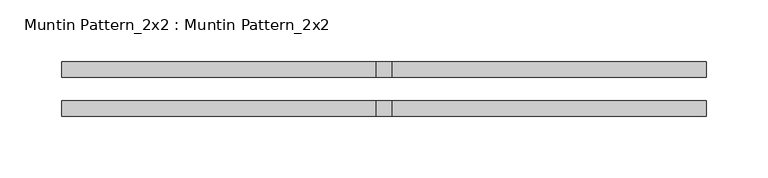
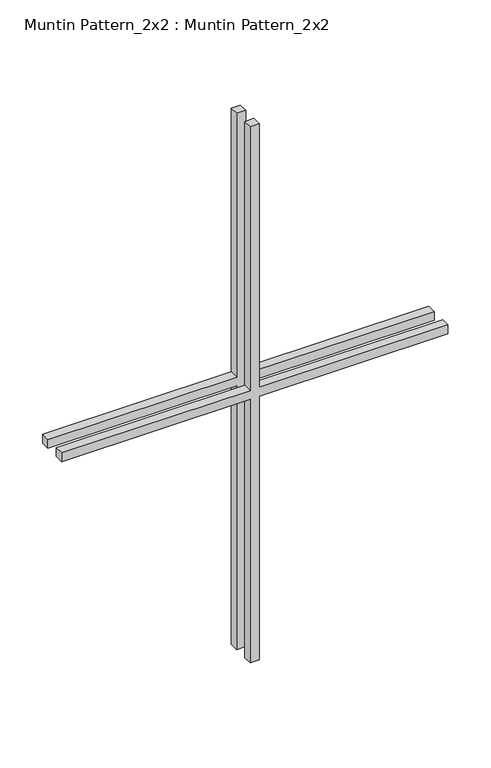
"""IFC4 building model written with IfcOpenShell, lengths in millimetres: proxy geometry, Muntin Pattern_2x2 : Muntin Pattern_2x2."""

from ifc_helpers import new_model, si_unit, frame, origin, place, context, project, spatial, polyline, outline, extrude, source, transform, mapped, element, save


def muntin_pattern_2x2_muntin_pattern_2x2_1fb5fae3(model_context):
    return source(origin(), model_context, "Body", "SweptSolid", [
        extrude(outline(polyline([(390.525, -6.35), (390.525, -261.9375), (377.825, -261.9375), (377.825, -6.35), (0.0, -6.35), (0.0, 6.35), (377.825, 6.35), (377.825, 261.9375), (390.525, 261.9375), (390.525, 6.35), (768.35, 6.35), (768.35, -6.35), (390.525, -6.35)])), frame((0.0, -22.225, 0.0), z_axis=(0.0, 1.0, 0.0), x_axis=(0.0, 0.0, 1.0)), (0.0, 0.0, 1.0), 12.7),
        extrude(outline(polyline([(390.525, -6.35), (390.525, -261.9375), (377.825, -261.9375), (377.825, -6.35), (0.0, -6.35), (0.0, 6.35), (377.825, 6.35), (377.825, 261.9375), (390.525, 261.9375), (390.525, 6.35), (768.35, 6.35), (768.35, -6.35), (390.525, -6.35)])), frame((0.0, 9.525, 0.0), z_axis=(0.0, 1.0, 0.0), x_axis=(0.0, 0.0, 1.0)), (0.0, 0.0, 1.0), 12.7),
    ])


if __name__ == "__main__":
    model = new_model("IFC4")
    model_context = context("Model", 3, world=origin())
    ifc_project = project(units=[si_unit("LENGTHUNIT", "METRE", prefix="MILLI")], contexts=[model_context])
    site = spatial("IfcSite", under=ifc_project)
    building = spatial("IfcBuilding", under=site)
    placement = place(None, origin())
    muntin_pattern_2x2_muntin_pattern_2x2_shape = muntin_pattern_2x2_muntin_pattern_2x2_1fb5fae3(model_context)
    element("IfcBuildingElementProxy", 1, Name="Muntin Pattern_2x2 : Muntin Pattern_2x2", ObjectType="Muntin Pattern_2x2 : Muntin Pattern_2x2", at=placement, inside=building, context=model_context, shape_type="MappedRepresentation", body=[
        mapped(muntin_pattern_2x2_muntin_pattern_2x2_shape, transform((0.0, 0.0, 0.0), x_axis=(1.0, 0.0, 0.0), y_axis=(0.0, 1.0, 0.0), z_axis=(0.0, 0.0, 1.0))),
    ])
    save(model, "model.ifc")

# Revit data of these elements
# Type "Muntin Pattern_2x2 : Muntin Pattern_2x2"
#   Width [instance default] = 4' - 0"
#   Thickness = 0' - 0 1/2"
#   Height [instance default] = 4' - 0"
#   Distance = 0' - 0 3/4"
#   Interior Material [instance default] = none
#   Exterior Material [instance default] = none
#   Default Elevation = 0
# Element 1 (IfcBuildingElementProxy, "Muntin Pattern_2x2 : Muntin Pattern_2x2")
#   Width = 1' - 8 5/8"
#   Height = 2' - 6 1/4"
#   Interior Material = Wood - Stained
#   Exterior Material = Clad - White
#   Materials on its faces: "Clad - White", "Wood - Stained"
# Materials
#   "Clad - White": class "Wood", colour RGB 242 242 238, transparency 0, Cost = 0
#   "Wood - Stained": class "Wood", colour RGB 224 178 126, transparency 0, Cost = 0
